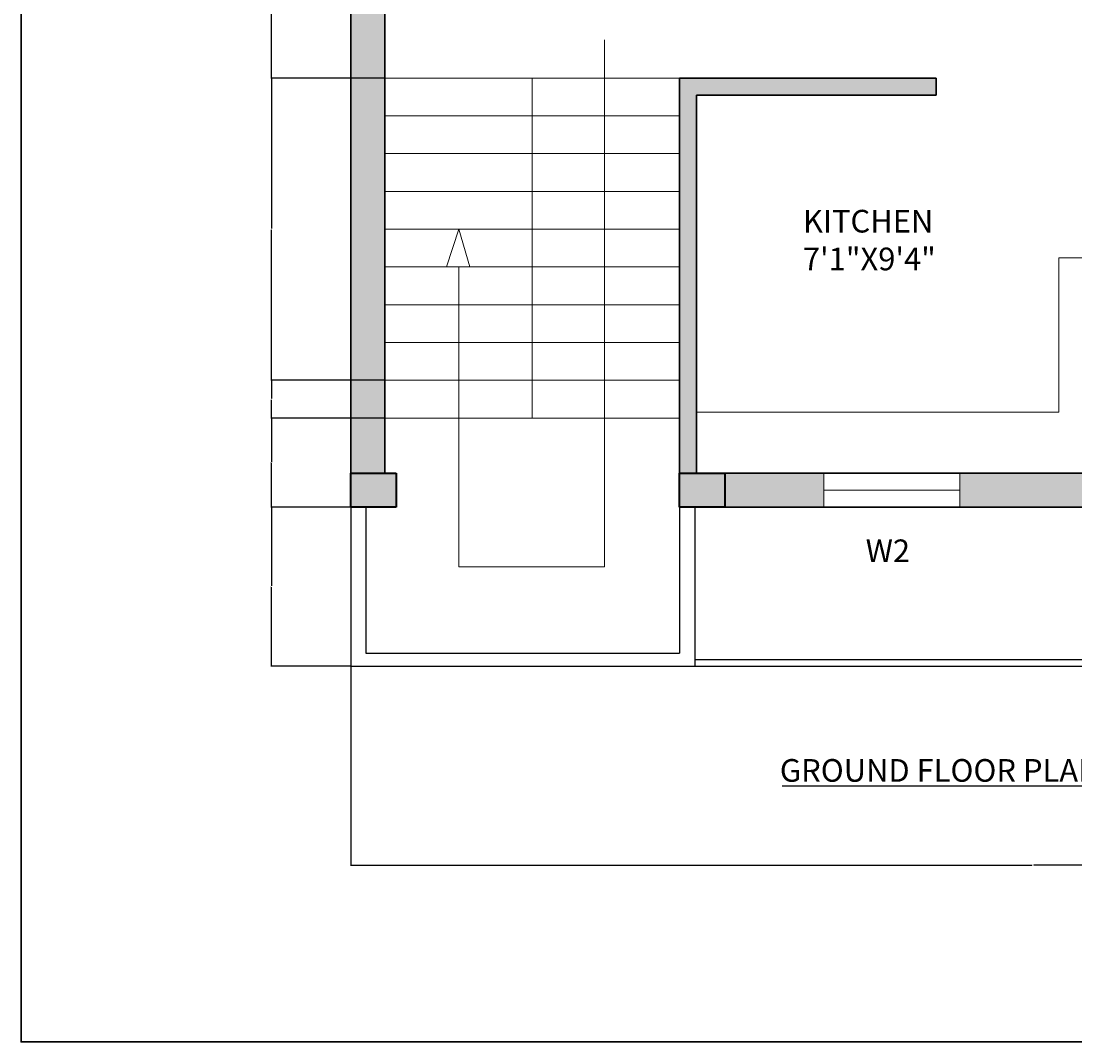
# Model space of a CAD drawing. Units: inches. Extents: x 1623 to 2200, y 2019 to 3010.
# Tile 1 of 6: x 1623 to 1902, y 2019 to 2290. Entities that reach past the tile are written whole.
import ezdxf

# ---------------------------------------------------------------- set-up
doc = ezdxf.new("R2010")
doc.units = ezdxf.units.IN
for name, color, linetype, lineweight in [('A-ANNO-DIMS', 2, 'Continuous', 18), ('A-ANNO-TITL', 7, 'Continuous', 25), ('A-ANNO-TTLB', 7, 'Continuous', 35), ('A-AREA-IDEN', 7, 'Continuous', 18), ('A-COLS', 7, 'Continuous', 40), ('A-FLOR-BALC', 7, 'Continuous', 25), ('A-FLOR-CASE', 8, 'Continuous', 18), ('A-FLOR-STRS', 7, 'Continuous', 18), ('A-GLAZ', 4, 'Continuous', 18), ('A-GLAZ-IDEN', 7, 'Continuous', 18), ('A-WALL', 7, 'Continuous', 35)]:
    doc.layers.add(name, color=color, linetype=linetype, lineweight=lineweight)
doc.layers.add('A-COLS-PATT', color=152, linetype='Continuous', lineweight=13, true_color=0x2776bb)
doc.layers.add('A-WALL-PATT', color=251, linetype='Continuous', lineweight=13, true_color=0x636466)
doc.styles.get("Standard").update_dxf_attribs({"font": 'arial.ttf'})
doc.dimstyles.get("Standard").update_dxf_attribs({"dimtxt": 0.18, "dimasz": 0.18, "dimexe": 0.18, "dimexo": 0.0625, "dimgap": 0.09, "dimtad": 0, "dimtih": 1, "dimtoh": 1, "dimdec": 4, "dimzin": 0, "dimdsep": 46, "dimtxsty": 'Standard', "dimcen": 0.09, "dimadec": 0, "dimazin": 0, "dimtfac": 1, "dimtdec": 4, "dimtofl": 0, "dimtmove": 0, "dimatfit": 3, "dimfxl": 1, "dimtolj": 1, "dimtzin": 0, "dimarcsym": 0})

# ---------------------------------------------------------------- blocks, each defined once
blk = doc.blocks.new('COL-12X9-PLAN')
for p, q in [((0, 0), (0, 9)), ((0, 9), (12, 9)), ((12, 9), (12, 0)), ((9, 0), (0, 0)), ((12, 0), (9, 0))]:
    blk.add_line(p, q)
blk = doc.blocks.new('*D28')
at = {"layer": 'A-ANNO-DIMS', "color": 0, "lineweight": -2, "transparency": 16777216}
for p, q in [((1710.33, 2118.83), (1710.33, 2066.05)), ((2071.33, 2118.83), (2071.33, 2066.05)), ((1710.51, 2066.23), (1890.55, 2066.23)), ((2071.15, 2066.23), (1891.1, 2066.23))]:
    blk.add_line(p, q, dxfattribs=at)
at = {"layer": 'A-ANNO-DIMS', "color": 0, "transparency": 16777216}
for points in [[(1710.51, 2066.26), (1710.51, 2066.2), (1710.33, 2066.23)], [(2071.15, 2066.26), (2071.15, 2066.2), (2071.33, 2066.23)]]:
    blk.add_solid(points, dxfattribs=at)
at = {"layer": 'Defpoints', "color": 0, "transparency": 16777216}
for p in [(1710.33, 2118.89), (2071.33, 2118.89), (2071.33, 2066.23)]:
    blk.add_point(p, dxfattribs=at)
at = {"layer": 'A-ANNO-DIMS', "color": 0, "transparency": 16777216, "insert": (1890.83, 2066.23), "char_height": 0.18, "attachment_point": 5}
blk.add_mtext('\\A1;361', dxfattribs=at)
blk = doc.blocks.new('*D37')
at = {"layer": 'A-ANNO-DIMS', "color": 0, "lineweight": -2, "transparency": 16777216}
for p, q in [((1710.26, 2161.02), (1689.17, 2161.02)), ((1689.35, 2160.84), (1689.35, 2140.14)), ((1689.35, 2119.07), (1689.35, 2139.78)), ((1710.26, 2118.89), (1689.17, 2118.89))]:
    blk.add_line(p, q, dxfattribs=at)
at = {"layer": 'A-ANNO-DIMS', "color": 0, "transparency": 16777216}
for points in [[(1689.32, 2160.84), (1689.38, 2160.84), (1689.35, 2161.02)], [(1689.32, 2119.07), (1689.38, 2119.07), (1689.35, 2118.89)]]:
    blk.add_solid(points, dxfattribs=at)
at = {"layer": 'Defpoints', "color": 0, "transparency": 16777216}
for p in [(1689.35, 2161.02), (1710.33, 2161.02), (1710.33, 2118.89)]:
    blk.add_point(p, dxfattribs=at)
at = {"layer": 'A-ANNO-DIMS', "color": 0, "transparency": 16777216, "insert": (1689.35, 2139.96), "char_height": 0.18, "attachment_point": 5}
blk.add_mtext('\\A1;42.13', dxfattribs=at)
blk = doc.blocks.new('*D38')
at = {"layer": 'A-ANNO-DIMS', "color": 0, "lineweight": -2, "transparency": 16777216}
for p, q in [((1719.26, 2184.59), (1689.17, 2184.59)), ((1689.35, 2184.41), (1689.35, 2172.99)), ((1689.35, 2161.2), (1689.35, 2172.63)), ((1710.26, 2161.02), (1689.17, 2161.02))]:
    blk.add_line(p, q, dxfattribs=at)
at = {"layer": 'A-ANNO-DIMS', "color": 0, "transparency": 16777216}
for points in [[(1689.32, 2184.41), (1689.38, 2184.41), (1689.35, 2184.59)], [(1689.32, 2161.2), (1689.38, 2161.2), (1689.35, 2161.02)]]:
    blk.add_solid(points, dxfattribs=at)
at = {"layer": 'Defpoints', "color": 0, "transparency": 16777216}
for p in [(1689.35, 2184.59), (1719.33, 2184.59), (1710.33, 2161.02)]:
    blk.add_point(p, dxfattribs=at)
at = {"layer": 'A-ANNO-DIMS', "color": 0, "transparency": 16777216, "insert": (1689.35, 2172.81), "char_height": 0.18, "attachment_point": 5}
blk.add_mtext('\\A1;23.57', dxfattribs=at)
blk = doc.blocks.new('*D39')
at = {"layer": 'A-ANNO-DIMS', "color": 0, "lineweight": -2, "transparency": 16777216}
for p, q in [((1719.26, 2194.59), (1689.17, 2194.59)), ((1689.35, 2194.41), (1689.35, 2189.78)), ((1689.35, 2184.77), (1689.35, 2189.41)), ((1719.26, 2184.59), (1689.17, 2184.59))]:
    blk.add_line(p, q, dxfattribs=at)
at = {"layer": 'A-ANNO-DIMS', "color": 0, "transparency": 16777216}
for points in [[(1689.32, 2194.41), (1689.38, 2194.41), (1689.35, 2194.59)], [(1689.32, 2184.77), (1689.38, 2184.77), (1689.35, 2184.59)]]:
    blk.add_solid(points, dxfattribs=at)
at = {"layer": 'Defpoints', "color": 0, "transparency": 16777216}
for p in [(1689.35, 2194.59), (1719.33, 2194.59), (1719.33, 2184.59)]:
    blk.add_point(p, dxfattribs=at)
at = {"layer": 'A-ANNO-DIMS', "color": 0, "transparency": 16777216, "insert": (1689.35, 2189.59), "char_height": 0.18, "attachment_point": 5}
blk.add_mtext('\\A1;10', dxfattribs=at)
blk = doc.blocks.new('*D40')
at = {"layer": 'A-ANNO-DIMS', "color": 0, "lineweight": -2, "transparency": 16777216}
for p, q in [((1719.26, 2274.59), (1689.17, 2274.59)), ((1689.35, 2274.41), (1689.35, 2234.78)), ((1689.35, 2194.77), (1689.35, 2234.41)), ((1719.26, 2194.59), (1689.17, 2194.59))]:
    blk.add_line(p, q, dxfattribs=at)
at = {"layer": 'A-ANNO-DIMS', "color": 0, "transparency": 16777216}
for points in [[(1689.32, 2274.41), (1689.38, 2274.41), (1689.35, 2274.59)], [(1689.32, 2194.77), (1689.38, 2194.77), (1689.35, 2194.59)]]:
    blk.add_solid(points, dxfattribs=at)
at = {"layer": 'Defpoints', "color": 0, "transparency": 16777216}
for p in [(1689.35, 2274.59), (1719.33, 2274.59), (1719.33, 2194.59)]:
    blk.add_point(p, dxfattribs=at)
at = {"layer": 'A-ANNO-DIMS', "color": 0, "transparency": 16777216, "insert": (1689.35, 2234.59), "char_height": 0.18, "attachment_point": 5}
blk.add_mtext('\\A1;80', dxfattribs=at)
blk = doc.blocks.new('*D41')
at = {"layer": 'A-ANNO-DIMS', "color": 0, "lineweight": -2, "transparency": 16777216}
for p, q in [((1710.26, 2342.02), (1689.17, 2342.02)), ((1689.35, 2341.84), (1689.35, 2308.49)), ((1689.35, 2274.77), (1689.35, 2308.13)), ((1719.26, 2274.59), (1689.17, 2274.59))]:
    blk.add_line(p, q, dxfattribs=at)
at = {"layer": 'A-ANNO-DIMS', "color": 0, "transparency": 16777216}
for points in [[(1689.32, 2341.84), (1689.38, 2341.84), (1689.35, 2342.02)], [(1689.32, 2274.77), (1689.38, 2274.77), (1689.35, 2274.59)]]:
    blk.add_solid(points, dxfattribs=at)
at = {"layer": 'Defpoints', "color": 0, "transparency": 16777216}
for p in [(1689.35, 2342.02), (1710.32, 2342.02), (1719.33, 2274.59)]:
    blk.add_point(p, dxfattribs=at)
at = {"layer": 'A-ANNO-DIMS', "color": 0, "transparency": 16777216, "insert": (1689.35, 2308.31), "char_height": 0.18, "attachment_point": 5}
blk.add_mtext('\\A1;67.43', dxfattribs=at)

msp = doc.modelspace()

# ---------------------------------------------------------------- hatches: boundary and pattern name
at = {"layer": 'A-COLS-PATT'}
h = msp.add_hatch(color=256, dxfattribs=at)
h.dxf.hatch_style = 1
h.paths.add_polyline_path([(1722.3258, 2483.5237), (1710.3258, 2483.5237), (1710.3258, 2474.5237), (1719.3258, 2474.5237), (1722.3258, 2474.5237)])
h.paths.add_polyline_path([(1809.3258, 2483.5237), (1797.3258, 2483.5237), (1797.3258, 2474.5237), (1806.3258, 2474.5237), (1809.3258, 2474.5237)])
h.paths.add_polyline_path([(1918.3972, 2483.5237), (1906.3972, 2483.5237), (1906.3972, 2474.5237), (1915.3972, 2474.5237), (1918.3972, 2474.5237)])
h.paths.add_polyline_path([(2071.3258, 2483.5237), (2059.3258, 2483.5237), (2059.3258, 2474.532), (2068.3258, 2474.532), (2071.3258, 2474.532)])
h.paths.add_polyline_path([(2071.3258, 2351.0312), (2059.3258, 2351.0312), (2059.3258, 2342.0312), (2068.3258, 2342.0312), (2071.3258, 2342.0312)])
h.paths.add_polyline_path([(1918.3258, 2351.0237), (1906.3258, 2351.0237), (1906.3258, 2342.0237), (1915.3258, 2342.0237), (1918.3258, 2342.0237)])
h.paths.add_polyline_path([(1722.3198, 2351.0237), (1710.3258, 2351.0237), (1710.3258, 2342.0237), (1719.3198, 2342.0237), (1722.3198, 2342.0237)])
h.paths.add_polyline_path([(1809.3158, 2351.0237), (1797.3258, 2351.0237), (1797.3258, 2346.5237), (1797.3158, 2342.0237), (1806.3158, 2342.0237), (1809.3158, 2342.0237)])
h.paths.add_polyline_path([(1722.3029, 2170.0237), (1710.3258, 2170.0237), (1710.3258, 2161.0237), (1714.3029, 2161.0237), (1719.3029, 2161.0237), (1722.3029, 2161.0237)])
h.paths.add_polyline_path([(1809.3258, 2170.0237), (1797.3258, 2170.0237), (1797.3258, 2161.0237), (1801.3258, 2161.0237), (1802.9141, 2161.0237), (1806.3258, 2161.0237), (1809.3258, 2161.0237)])
h.paths.add_polyline_path([(1918.2273, 2170.0237), (1906.2273, 2170.0237), (1906.2273, 2161.0237), (1915.2273, 2161.0237), (1918.2273, 2161.0237)])
h.paths.add_polyline_path([(2071.3258, 2170.0237), (2059.3258, 2170.0237), (2059.3258, 2161.0237), (2068.3258, 2161.0237), (2071.3258, 2161.0237)])
at = {"layer": 'A-WALL-PATT'}
h = msp.add_hatch(color=256, dxfattribs=at)
h.dxf.hatch_style = 1
h.paths.add_polyline_path([(1725.9857, 2483.5237), (1722.3258, 2483.5237), (1722.3258, 2474.5237), (1725.9857, 2474.5237), (1725.9857, 2479.0237)])
h.paths.add_polyline_path([(1797.3258, 2483.5237), (1749.9857, 2483.5237), (1749.9857, 2474.5237), (1797.3258, 2474.5237)])
h.paths.add_polyline_path([(1830.4977, 2483.5237), (1809.3258, 2483.5237), (1809.3258, 2474.5237), (1830.4977, 2474.5237), (1830.4977, 2479.0237)])
h.paths.add_polyline_path([(1906.3972, 2483.5237), (1878.4977, 2483.5237), (1878.4977, 2474.5237), (1906.3972, 2474.5237)])
h.paths.add_polyline_path([(1918.3258, 2474.5237), (1915.3972, 2474.5237), (1913.8258, 2474.5237), (1913.8258, 2395.0237), (1913.8258, 2384.7587), (1918.3258, 2384.7587), (1918.3258, 2395.0237)])
h.paths.add_polyline_path([(1801.8258, 2474.5237), (1797.3258, 2474.5237), (1797.3258, 2436.0951), (1801.8258, 2436.0951)], flags=17)
h.paths.add_polyline_path([(1719.3258, 2474.5237), (1710.3258, 2474.5237), (1710.3258, 2351.0237), (1719.3258, 2351.0237), (1719.3258, 2395.0237), (1801.8258, 2395.0237), (1801.8258, 2399.5237), (1719.3258, 2399.5237)])
h.paths.add_polyline_path([(1797.3158, 2346.5237), (1722.3198, 2346.5237), (1722.3198, 2342.0237), (1797.3158, 2342.0237)])
h.paths.add_polyline_path([(1801.8258, 2361.4421), (1797.3258, 2361.4421), (1797.3258, 2351.0237), (1801.8258, 2351.0237)], flags=17)
h.paths.add_polyline_path([(2059.3258, 2346.5237), (1918.3258, 2346.5237), (1918.3258, 2342.0237), (2059.3258, 2342.0237)])
h.paths.add_polyline_path([(1963.26, 2479.0237), (1963.26, 2483.5237), (1918.3972, 2483.5237), (1918.3972, 2474.5237), (1963.26, 2474.5237)])
h.paths.add_polyline_path([(2059.3258, 2483.5237), (2011.26, 2483.5237), (2011.26, 2474.5237), (2059.3258, 2474.5237)])
h.paths.add_polyline_path([(2071.3258, 2474.532), (2068.3258, 2474.532), (2062.3258, 2474.532), (2062.3258, 2351.0312), (2071.3258, 2351.0312)])
h.paths.add_polyline_path([(2071.3258, 2342.0312), (2068.3258, 2342.0312), (2062.3258, 2342.0312), (2062.3258, 2170.0237), (2071.3258, 2170.0237)])
h.paths.add_polyline_path([(2059.3258, 2170.0237), (2038.3258, 2170.0237), (2038.3258, 2161.0237), (2059.3258, 2161.0237)])
h.paths.add_polyline_path([(1990.3258, 2170.0237), (1963.4402, 2170.0237), (1963.4402, 2161.0237), (1990.3258, 2161.0237), (1990.3258, 2165.5237)])
h.paths.add_polyline_path([(1918.3258, 2274.595), (1913.8258, 2274.595), (1913.8258, 2170.0237), (1918.3258, 2170.0237)])
h.paths.add_polyline_path([(1906.2273, 2170.0237), (1871.454, 2170.0237), (1871.454, 2161.0237), (1906.2273, 2161.0237)])
h.paths.add_polyline_path([(1835.454, 2170.0237), (1809.3258, 2170.0237), (1809.3258, 2161.0237), (1835.454, 2161.0237), (1835.454, 2165.5237)])
h.paths.add_polyline_path([(1801.8258, 2270.095), (1865.2406, 2270.095), (1865.2406, 2274.595), (1797.3258, 2274.595), (1797.3258, 2170.0237), (1801.8258, 2170.0237)])
h.paths.add_polyline_path([(1719.3258, 2342.0237), (1719.3198, 2342.0237), (1710.3258, 2342.0237), (1710.3258, 2170.0237), (1719.3258, 2170.0237)])

# ---------------------------------------------------------------- linework, layer by layer
at = {"layer": 'A-ANNO-TITL'}
msp.add_line((1824.4388, 2087.1806), (1915.7543, 2087.1806), dxfattribs=at)
at = {"layer": 'A-ANNO-TTLB'}
msp.add_lwpolyline([(1623.0453, 3010.4913), (2200.0052, 3010.4913), (2200.0052, 2019.4245), (1623.0453, 2019.4245)], close=True, dxfattribs=at)
at = {"layer": 'A-FLOR-BALC'}
for p, q in [((1710.3029, 2161.0237), (1714.3029, 2161.0237)), ((1710.3258, 2161.0237), (1710.3258, 2118.8921)), ((1714.3029, 2161.0237), (1714.3029, 2122.3414)), ((1797.3258, 2161.0237), (1797.3258, 2122.3414)), ((1797.3258, 2161.0237), (1802.9141, 2161.0237)), ((1797.3258, 2161.0237), (1801.3258, 2161.0237)), ((1801.3258, 2161.0237), (1801.3258, 2118.8921)), ((1714.3029, 2122.3414), (1797.3258, 2122.3414)), ((1797.3258, 2122.3414), (1797.3258, 2122.3414)), ((2069.3258, 2120.5833), (1801.3258, 2120.5833)), ((1710.3258, 2118.8921), (1714.8258, 2118.8921)), ((1714.8258, 2118.8921), (2071.3258, 2118.8921))]:
    msp.add_line(p, q, dxfattribs=at)
at = {"layer": 'A-FLOR-CASE'}
for p, q in [((1897.6607, 2186.1489), (1897.6607, 2227.0114)), ((1897.6607, 2227.0114), (1913.8258, 2227.0114)), ((1801.8258, 2186.1489), (1897.6607, 2186.1489))]:
    msp.add_line(p, q, dxfattribs=at)
at = {"layer": 'A-FLOR-STRS'}
for p, q in [((1777.4149, 2284.7537), (1777.4149, 2145.2127)), ((1797.3258, 2274.595), (1719.3258, 2274.595)), ((1758.3258, 2274.595), (1758.3258, 2184.595)), ((1797.3258, 2264.595), (1719.3258, 2264.595)), ((1797.3258, 2254.595), (1719.3258, 2254.595)), ((1797.3258, 2244.595), (1719.3258, 2244.595)), ((1797.3258, 2234.595), (1719.3258, 2234.595)), ((1738.8592, 2234.595), (1735.6625, 2224.595)), ((1741.8437, 2224.595), (1738.8592, 2234.595)), ((1797.3258, 2224.595), (1719.3258, 2224.595)), ((1735.6625, 2224.595), (1741.8437, 2224.595)), ((1738.8592, 2145.2127), (1738.8592, 2224.595)), ((1797.3258, 2214.595), (1719.3258, 2214.595)), ((1797.3258, 2204.595), (1719.3258, 2204.595)), ((1797.3258, 2194.595), (1719.3258, 2194.595)), ((1797.3258, 2184.595), (1719.3258, 2184.595)), ((1777.4149, 2145.2127), (1738.8592, 2145.2127))]:
    msp.add_line(p, q, dxfattribs=at)
at = {"layer": 'A-GLAZ'}
for p, q in [((1835.454, 2170.0237), (1835.454, 2161.0237)), ((1871.454, 2165.5237), (1871.454, 2170.0237)), ((1871.454, 2170.0237), (1871.454, 2161.0237)), ((1835.454, 2161.0237), (1835.454, 2165.5237)), ((1835.454, 2165.5237), (1835.454, 2165.5237)), ((1835.454, 2165.5237), (1871.454, 2165.5237))]:
    msp.add_line(p, q, dxfattribs=at)
at = {"layer": 'A-WALL'}
for p, q in [((1710.3258, 2483.5237), (1710.3258, 2161.0237)), ((1719.3258, 2342.0237), (1719.3258, 2170.0237)), ((1865.2406, 2274.595), (1797.3258, 2274.595)), ((1797.3258, 2274.595), (1797.3258, 2170.0237)), ((1865.2406, 2270.095), (1865.2406, 2274.595)), ((1801.8258, 2270.095), (1865.2406, 2270.095)), ((1801.8258, 2270.095), (1801.8258, 2170.0237)), ((1719.3258, 2170.0237), (1722.3029, 2170.0237)), ((1801.8258, 2170.0237), (1913.8258, 2170.0237)), ((1710.3258, 2161.0237), (1722.3029, 2161.0237)), ((1797.3258, 2161.0237), (1918.2273, 2161.0237))]:
    msp.add_line(p, q, dxfattribs=at)

# ---------------------------------------------------------------- block references
at = {"layer": 'A-COLS'}
for p in [(1710.3031, 2161.024), (1797.326, 2161.024)]:
    msp.add_blockref('COL-12X9-PLAN', p, dxfattribs=at)

# ---------------------------------------------------------------- texts
at = {"layer": 'A-ANNO-TITL', "insert": (1823.8511, 2094.305), "char_height": 6, "attachment_point": 1}
msp.add_mtext_dynamic_manual_height_columns('GROUND FLOOR PLAN', width=316.739638, gutter_width=12.5, heights=[0], dxfattribs=at)
at = {"layer": 'A-AREA-IDEN', "insert": (1829.953, 2239.7035), "char_height": 6, "attachment_point": 1}
msp.add_mtext_dynamic_manual_height_columns('KITCHEN\\P7\'1"X9\'4"', width=96.210898, gutter_width=12.5, heights=[0], dxfattribs=at)
at = {"layer": 'A-GLAZ-IDEN', "insert": (1846.5792, 2152.437), "char_height": 6, "attachment_point": 1}
msp.add_mtext_dynamic_manual_height_columns('W2', width=54.397259, gutter_width=12.5, heights=[0], dxfattribs=at)

# ---------------------------------------------------------------- dimensions: what is measured, and where the dimension line sits
at = {"layer": 'A-ANNO-DIMS'}
for base, p1, p2, override, picture, middle in [((1689.3529, 2342.0237), (1719.3258, 2274.595), (1710.3198, 2342.0237), {"dimdec": 2, "dimlfac": 1, "dimrnd": 0, "dimzin": 0, "dimdsep": 46, "dimlunit": 2}, '*D41', (1689.3529, 2308.3093)), ((1689.3529, 2274.595), (1719.3258, 2194.595), (1719.3258, 2274.595), {"dimdec": 0, "dimlfac": 1, "dimrnd": 0, "dimzin": 0, "dimdsep": 46, "dimlunit": 2}, '*D40', (1689.3529, 2234.595)), ((1689.3529, 2194.595), (1719.3258, 2184.595), (1719.3258, 2194.595), {"dimdec": 0, "dimlfac": 1, "dimrnd": 0, "dimzin": 0, "dimdsep": 46, "dimlunit": 2}, '*D39', (1689.3529, 2189.595)), ((1689.3529, 2184.595), (1710.3258, 2161.0237), (1719.3258, 2184.595), {"dimdec": 2, "dimlfac": 1, "dimrnd": 0, "dimzin": 0, "dimdsep": 46, "dimlunit": 2}, '*D38', (1689.3529, 2172.8093)), ((1689.3529, 2161.0237), (1710.3258, 2118.8921), (1710.3258, 2161.0237), {"dimdec": 2, "dimlfac": 1, "dimrnd": 0, "dimzin": 0, "dimdsep": 46, "dimlunit": 2}, '*D37', (1689.3529, 2139.9579))]:
    dim = msp.add_linear_dim(base=base, p1=p1, p2=p2, angle=90, dimstyle='Standard', override=override, dxfattribs=at)
    dim.commit()
    dim.dimension.update_dxf_attribs({"geometry": picture, "text_midpoint": middle})
dim = msp.add_linear_dim(base=(2071.3258, 2066.2306), p1=(1710.3258, 2118.8921), p2=(2071.3258, 2118.8921), dimstyle='Standard', override={"dimdec": 0, "dimlfac": 1, "dimrnd": 0, "dimzin": 0, "dimdsep": 46, "dimlunit": 2}, dxfattribs=at)
dim.commit()
dim.dimension.update_dxf_attribs({"geometry": '*D28', "text_midpoint": (1890.8258, 2066.2306)})

doc.saveas('drawing.dxf')
